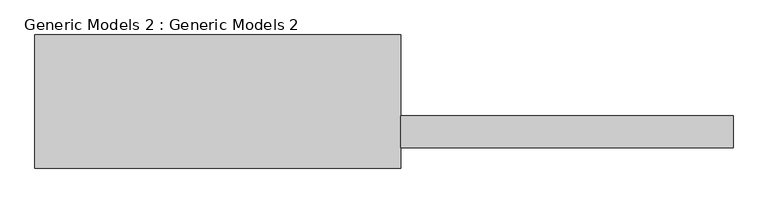
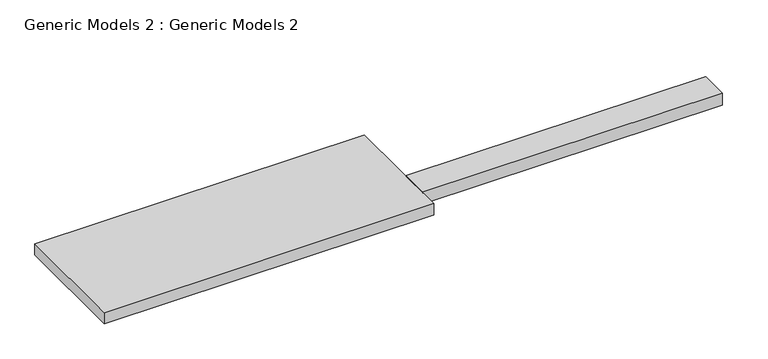
"""IFC4 building model written with IfcOpenShell, lengths in millimetres: proxy geometry, Generic Models 2 : Generic Models 2."""

from ifc_helpers import new_model, si_unit, origin, origin_with_axes, place, context, project, spatial, polyline, outline, extrude, source, transform, mapped, element, save


def generic_models_2_generic_models_2_78c8f357(model_context):
    return source(origin(), model_context, "Body", "SweptSolid", [
        extrude(outline(polyline([(-17585.2518575, -16985.2511694), (-17585.2518575, -15154.7378384), (-12556.0518575, -15154.7378384), (-12556.0518575, -16985.2511694), (-17585.2518575, -16985.2511694)])), origin_with_axes(), (0.0, 0.0, 1.0), 177.8),
        extrude(outline(polyline([(-7984.0518575, -16704.1816871), (-12556.0518575, -16704.1816871), (-12556.0518575, -16266.353918), (-7984.0518575, -16266.353918), (-7984.0518575, -16704.1816871)])), origin_with_axes(), (0.0, 0.0, 1.0), 195.9245847),
    ])


if __name__ == "__main__":
    model = new_model("IFC4")
    model_context = context("Model", 3, world=origin())
    ifc_project = project(units=[si_unit("LENGTHUNIT", "METRE", prefix="MILLI")], contexts=[model_context])
    site = spatial("IfcSite", under=ifc_project)
    building = spatial("IfcBuilding", under=site)
    placement = place(None, origin())
    generic_models_2_generic_models_2_shape = generic_models_2_generic_models_2_78c8f357(model_context)
    element("IfcBuildingElementProxy", 1, Name="Generic Models 2 : Generic Models 2", ObjectType="Generic Models 2 : Generic Models 2", at=placement, inside=building, context=model_context, shape_type="MappedRepresentation", body=[
        mapped(generic_models_2_generic_models_2_shape, transform((0.0, 0.0, 0.0), x_axis=(1.0, 0.0, 0.0), y_axis=(0.0, 1.0, 0.0), z_axis=(0.0, 0.0, 1.0))),
    ])
    save(model, "model.ifc")
